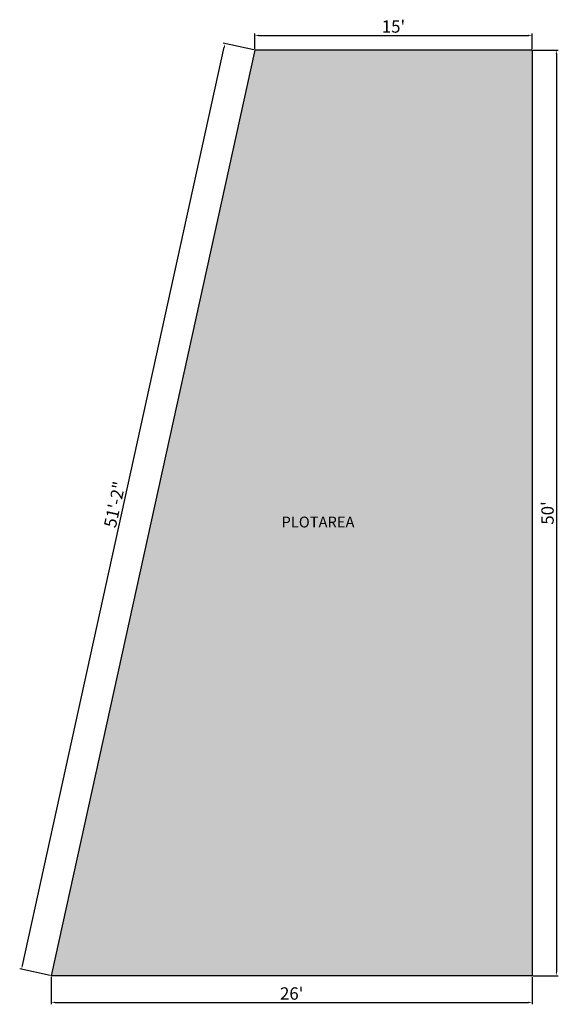
# Model space of a CAD drawing. Units: inches. Extents: x 2642 to 4124, y 1227 to 1973.
# Tile 7 of 7: x 3775 to 4124, y 1289 to 1927. Entities that reach past the tile are written whole.
import ezdxf

# ---------------------------------------------------------------- set-up
doc = ezdxf.new("R2010")
doc.units = ezdxf.units.IN
for name, color, linetype, lineweight in [('A-ANNO-DIMS', 2, 'Continuous', 18), ('A-AREA-IDEN', 7, 'Continuous', 18), ('C-PROP', 7, 'Continuous', 25)]:
    doc.layers.add(name, color=color, linetype=linetype, lineweight=lineweight)
doc.layers.add('C-PROP-PATT', color=9, linetype='Continuous', lineweight=13, true_color=0xc7c8ca)
doc.styles.get("Standard").update_dxf_attribs({"font": 'arial.ttf'})
doc.dimstyles.new('ISO-25', dxfattribs={"dimtxt": 8, "dimasz": 2.5, "dimexe": 1.25, "dimexo": 0.625, "dimtad": 1, "dimdec": 0, "dimlunit": 3, "dimtxsty": 'Standard', "dimcen": 2.5, "dimadec": 0, "dimazin": 0, "dimtfac": 1, "dimtdec": 0, "dimtmove": 0, "dimatfit": 3, "dimfxl": 1, "dimarcsym": 0})

# ---------------------------------------------------------------- blocks, each defined once
blk = doc.blocks.new('*D7')
at = {"layer": 'A-ANNO-DIMS', "color": 0, "lineweight": -2, "transparency": 16777216}
for p, q in [((3927.15, 1908.41), (3927.15, 1918.57)), ((3929.65, 1917.32), (4104.65, 1917.32)), ((4107.15, 1908.41), (4107.15, 1918.57))]:
    blk.add_line(p, q, dxfattribs=at)
at = {"layer": 'A-ANNO-DIMS', "color": 0, "transparency": 16777216}
for points in [[(3929.65, 1917.74), (3929.65, 1916.9), (3927.15, 1917.32)], [(4104.65, 1917.74), (4104.65, 1916.9), (4107.15, 1917.32)]]:
    blk.add_solid(points, dxfattribs=at)
at = {"layer": 'Defpoints', "color": 0, "transparency": 16777216}
for p in [(4107.15, 1917.32), (3927.15, 1907.78), (4107.15, 1907.78)]:
    blk.add_point(p, dxfattribs=at)
at = {"layer": 'A-ANNO-DIMS', "color": 0, "transparency": 16777216, "insert": (4017.15, 1922.03), "char_height": 8, "attachment_point": 5}
blk.add_mtext("15'", dxfattribs=at)
blk = doc.blocks.new('*D8')
at = {"layer": 'A-ANNO-DIMS', "color": 0, "lineweight": -2, "transparency": 16777216}
for p, q in [((4107.77, 1907.78), (4124.06, 1907.78)), ((4122.81, 1905.28), (4122.81, 1310.28)), ((4107.77, 1307.78), (4124.06, 1307.78))]:
    blk.add_line(p, q, dxfattribs=at)
at = {"layer": 'A-ANNO-DIMS', "color": 0, "transparency": 16777216}
for points in [[(4122.4, 1905.28), (4123.23, 1905.28), (4122.81, 1907.78)], [(4122.4, 1310.28), (4123.23, 1310.28), (4122.81, 1307.78)]]:
    blk.add_solid(points, dxfattribs=at)
at = {"layer": 'Defpoints', "color": 0, "transparency": 16777216}
for p in [(4107.15, 1907.78), (4107.15, 1307.78), (4122.81, 1307.78)]:
    blk.add_point(p, dxfattribs=at)
at = {"layer": 'A-ANNO-DIMS', "color": 0, "transparency": 16777216, "insert": (4118.1, 1607.78), "char_height": 8, "attachment_point": 5, "rotation": 90}
blk.add_mtext("50'", dxfattribs=at)
blk = doc.blocks.new('*D6')
at = {"layer": 'A-ANNO-DIMS', "color": 0, "lineweight": -2, "transparency": 16777216}
for p, q in [((3795.15, 1307.16), (3795.15, 1289.31)), ((4107.15, 1307.16), (4107.15, 1289.31)), ((3797.65, 1290.56), (4104.65, 1290.56))]:
    blk.add_line(p, q, dxfattribs=at)
at = {"layer": 'A-ANNO-DIMS', "color": 0, "transparency": 16777216}
for points in [[(3797.65, 1290.98), (3797.65, 1290.14), (3795.15, 1290.56)], [(4104.65, 1290.98), (4104.65, 1290.14), (4107.15, 1290.56)]]:
    blk.add_solid(points, dxfattribs=at)
at = {"layer": 'Defpoints', "color": 0, "transparency": 16777216}
for p in [(3795.15, 1307.78), (4107.15, 1307.78), (4107.15, 1290.56)]:
    blk.add_point(p, dxfattribs=at)
at = {"layer": 'A-ANNO-DIMS', "color": 0, "transparency": 16777216, "insert": (3951.15, 1295.27), "char_height": 8, "attachment_point": 5}
blk.add_mtext("26'", dxfattribs=at)
blk = doc.blocks.new('*D5')
at = {"layer": 'A-ANNO-DIMS', "color": 0, "lineweight": -2, "transparency": 16777216}
for p, q in [((3776.49, 1314.45), (3907.41, 1909.57)), ((3926.54, 1907.92), (3906.73, 1912.28)), ((3794.54, 1307.92), (3774.73, 1312.28))]:
    blk.add_line(p, q, dxfattribs=at)
at = {"layer": 'A-ANNO-DIMS', "color": 0, "transparency": 16777216}
for points in [[(3907.01, 1909.65), (3907.82, 1909.48), (3907.95, 1912.01)], [(3776.08, 1314.54), (3776.89, 1314.36), (3775.95, 1312.01)]]:
    blk.add_solid(points, dxfattribs=at)
at = {"layer": 'Defpoints', "color": 0, "transparency": 16777216}
for p in [(3907.95, 1912.01), (3927.15, 1907.78), (3795.15, 1307.78)]:
    blk.add_point(p, dxfattribs=at)
at = {"layer": 'A-ANNO-DIMS', "color": 0, "transparency": 16777216, "insert": (3837.35, 1613.02), "char_height": 8, "attachment_point": 5, "rotation": 77.59258}
blk.add_mtext('51\'-2"', dxfattribs=at)

msp = doc.modelspace()

# ---------------------------------------------------------------- hatches: boundary and pattern name
at = {"layer": 'C-PROP-PATT'}
h = msp.add_hatch(color=256, dxfattribs=at)
h.dxf.hatch_style = 1
h.paths.add_polyline_path([(4107.15, 1907.78), (3927.15, 1907.78), (3795.15, 1307.78), (4107.15, 1307.78)])
h.paths.add_polyline_path([(3942.61, 1594.41), (4000.09, 1594.41), (4000.09, 1609.35), (3942.61, 1609.35)], flags=24)

# ---------------------------------------------------------------- linework, layer by layer
at = {"layer": 'C-PROP'}
for p, q in [((3927.15, 1907.78), (3795.15, 1307.78)), ((4107.15, 1907.78), (3927.15, 1907.78)), ((4107.15, 1907.78), (4107.15, 1307.78)), ((4107.15, 1307.78), (3795.15, 1307.78))]:
    msp.add_line(p, q, dxfattribs=at)

# ---------------------------------------------------------------- texts
at = {"layer": 'A-AREA-IDEN', "insert": (3944.53, 1605.39), "char_height": 7, "attachment_point": 1}
msp.add_mtext_dynamic_manual_height_columns('{\\fTimes New Roman|b0|i0|c0|p18;PLOTAREA}', width=61.0557, gutter_width=12.5, heights=[0], dxfattribs=at)

# ---------------------------------------------------------------- dimensions: what is measured, and where the dimension line sits
at = {"layer": 'A-ANNO-DIMS'}
for base, p1, p2, picture, middle in [((4107.15, 1917.32), (3927.15, 1907.78), (4107.15, 1907.78), '*D7', (4017.15, 1922.03)), ((4107.15, 1290.56), (3795.15, 1307.78), (4107.15, 1307.78), '*D6', (3951.15, 1295.27))]:
    dim = msp.add_linear_dim(base=base, p1=p1, p2=p2, dimstyle='ISO-25', override={"dimclrd": 0, "dimclre": 0, "dimclrt": 0}, dxfattribs=at)
    dim.commit()
    dim.dimension.update_dxf_attribs({"geometry": picture, "text_midpoint": middle})
dim = msp.add_aligned_dim(p1=(3795.15, 1307.78), p2=(3927.15, 1907.78), distance=19.66, dimstyle='ISO-25', override={"dimclrd": 0, "dimclre": 0, "dimclrt": 0}, dxfattribs=at)
dim.commit()
dim.dimension.update_dxf_attribs({"geometry": '*D5', "text_midpoint": (3837.35, 1613.02)})
dim = msp.add_linear_dim(base=(4122.81, 1307.78), p1=(4107.15, 1907.78), p2=(4107.15, 1307.78), angle=90, dimstyle='ISO-25', override={"dimclrd": 0, "dimclre": 0, "dimclrt": 0}, dxfattribs=at)
dim.commit()
dim.dimension.update_dxf_attribs({"geometry": '*D8', "text_midpoint": (4118.1, 1607.78)})

doc.saveas('drawing.dxf')
